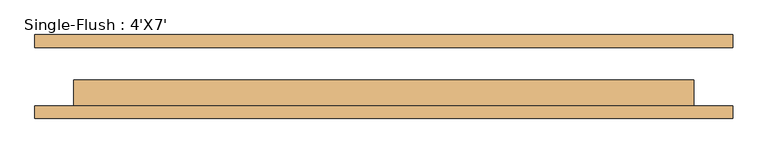
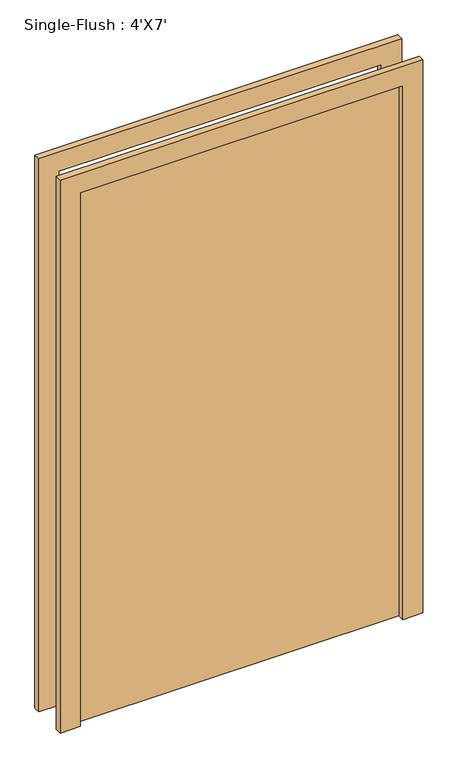
"""IFC4 building model written with IfcOpenShell, lengths in millimetres: door geometry, Single-Flush : 4'X7'."""

from ifc_helpers import new_model, si_unit, frame, origin, origin_with_axes, place, context, project, spatial, polyline, outline, extrude, source, transform, mapped, element, save


def single_flush_4_x7_9343de66(model_context):
    return source(origin(), model_context, "Body", "SweptSolid", [
        extrude(outline(polyline([(2209.8, -685.8), (0.0, -685.8), (0.0, -609.6), (2133.6, -609.6), (2133.6, 609.6), (0.0, 609.6), (0.0, 685.8), (2209.8, 685.8), (2209.8, -685.8)])), frame((0.0, -82.55, 0.0), z_axis=(0.0, 1.0, 0.0), x_axis=(0.0, 0.0, 1.0)), (0.0, 0.0, 1.0), 25.4),
        extrude(outline(polyline([(2209.8, 685.8), (2209.8, -685.8), (0.0, -685.8), (0.0, -609.6), (2133.6, -609.6), (2133.6, 609.6), (0.0, 609.6), (0.0, 685.8), (2209.8, 685.8)])), frame((0.0, 57.15, 0.0), z_axis=(0.0, 1.0, 0.0), x_axis=(0.0, 0.0, 1.0)), (0.0, 0.0, 1.0), 25.4),
        extrude(outline(polyline([(609.6, -6.35), (609.6, -57.15), (-609.6, -57.15), (-609.6, -6.35), (609.6, -6.35)])), origin_with_axes(), (0.0, 0.0, 1.0), 2133.6),
    ])


if __name__ == "__main__":
    model = new_model("IFC4")
    model_context = context("Model", 3, world=origin())
    ifc_project = project(units=[si_unit("LENGTHUNIT", "METRE", prefix="MILLI")], contexts=[model_context])
    site = spatial("IfcSite", under=ifc_project)
    building = spatial("IfcBuilding", under=site)
    placement = place(None, origin())
    single_flush_4_x7_shape = single_flush_4_x7_9343de66(model_context)
    element("IfcDoor", 1, ObjectType="Single-Flush : 4'X7'", at=placement, inside=building, context=model_context, shape_type="MappedRepresentation", body=[
        mapped(single_flush_4_x7_shape, transform((0.0, 0.0, 0.0), x_axis=(1.0, 0.0, 0.0), y_axis=(0.0, 1.0, 0.0), z_axis=(0.0, 0.0, 1.0))),
    ])
    save(model, "model.ifc")

# Revit data of these elements
# Type "Single-Flush : 4'X7'"
#   Type Mark = "12"
#   Construction Type Id = "MDOOR"
#   Assembly Code = "C1020"
#   Analytic Construction = "Metal"
#   Thickness = 0' - 2"
#   Heat Transfer Coefficient (U) = 0.651978 BTU/(h·ft²·°F)
#   Height = 7' - 0"
#   Trim Projection Ext = 0' - 1"
#   Trim Projection Int = 0' - 1"
#   Trim Width = 0' - 3"
#   Width = 4' - 0"
#   Define Thermal Properties by = 1
#   Door Material = Door - Panel
#   Frame Material = Door - Frame
#   Visual Light Transmittance = 0
#   Solar Heat Gain Coefficient = 0
#   Function = (empty or 0)
#   Wall Closure = (empty or 0)
# Element 1 (IfcDoor, "Single-Flush : 4'X7'")
#   Materials on its faces: "Door - Frame", "Door - Panel"
# Materials
#   "Door - Panel": class "Wood", colour RGB 210 159 95, transparency 0, Cost = 0
#   "Door - Frame": colour RGB 118 70 51, transparency 0, Cost = 0
